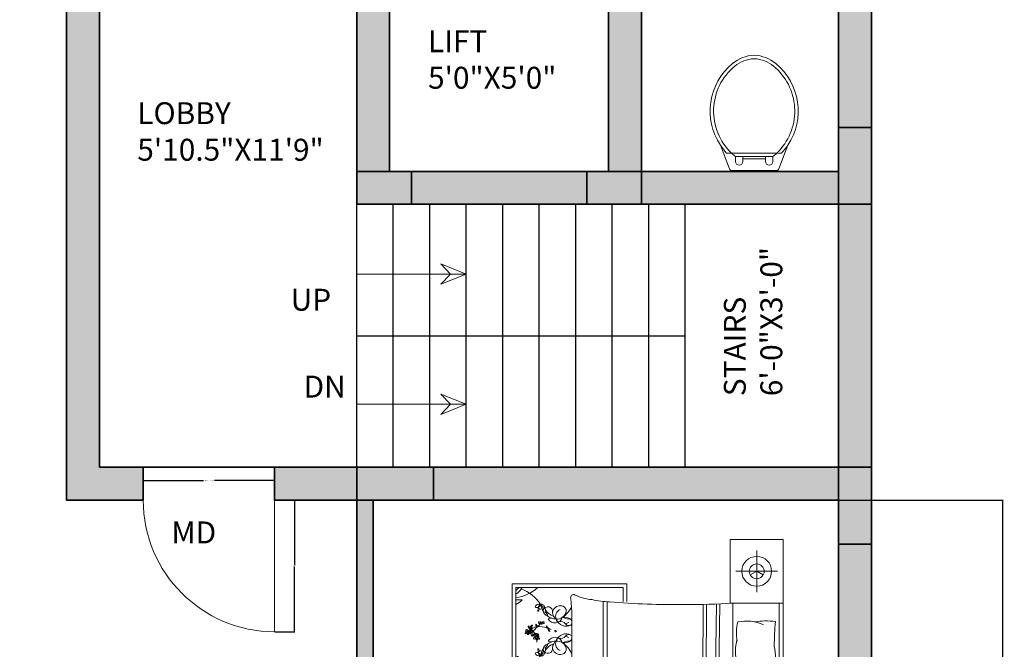
# Model space of a CAD drawing. Units: inches. Extents: x -9 to 505, y -680 to 48.
# Tile 6 of 17: x 235 to 505, y -487 to -314. Entities that reach past the tile are written whole.
import ezdxf

# ---------------------------------------------------------------- set-up
doc = ezdxf.new("R2010")
doc.units = ezdxf.units.IN
doc.header["$MEASUREMENT"] = 0
for name, color, linetype, lineweight in [('A-ANNO-DIMS', 2, 'Continuous', 18), ('A-ANNO-SYMB', 7, 'Continuous', 18), ('A-ANNO-TEXT', 7, 'Continuous', 18), ('A-AREA-IDEN', 7, 'Continuous', 18), ('A-DOOR', 3, 'Continuous', 18), ('A-FLOR-STRS', 7, 'Continuous', 25), ('A-FURN', 8, 'Continuous', 18), ('A-WALL', 7, 'Continuous', 35), ('A-WALL-PATT', 251, 'Continuous', 13), ('S-CONC', 7, 'Continuous', 35), ('S-CONC-PATT', 18, 'Continuous', 13), ('WC-Detail_dwgmodels.com', 251, 'Continuous', 13), ('WC-Outline_dwgmodels.com', 250, 'Continuous', 18)]:
    doc.layers.add(name, color=color, linetype=linetype, lineweight=lineweight)
doc.styles.get("Standard").update_dxf_attribs({"font": 'arial.ttf'})
doc.dimstyles.get("Standard").update_dxf_attribs({"dimtxt": 0.18, "dimasz": 0.18, "dimexe": 0.18, "dimexo": 0.0625, "dimgap": 0.09, "dimtad": 0, "dimtih": 1, "dimtoh": 1, "dimdec": 0, "dimzin": 0, "dimdsep": 46, "dimlunit": 3, "dimtxsty": 'Standard', "dimcen": 0.09, "dimadec": 0, "dimazin": 0, "dimtfac": 1, "dimtdec": 0, "dimtofl": 0, "dimtmove": 0, "dimatfit": 3, "dimfxl": 1, "dimtolj": 1, "dimtzin": 0, "dimarcsym": 0})

# ---------------------------------------------------------------- blocks, each defined once
blk = doc.blocks.new('BED-DOUBLE-WITH-NIGHTSTANDS')
for p, q in [((74.3, 0), (74.3, 87.37)), ((67.02, 72.93), (67.02, 84.34)), ((61.31, 78.63), (72.73, 78.63)), ((0, 75.23), (0, 11.53)), ((31.47, 75.23), (0, 75.23)), ((1.01, 74.22), (30.46, 74.22)), ((1.01, 12.54), (1.01, 74.22)), ((30.46, 74.22), (30.46, 70.37)), ((31.47, 70.38), (31.47, 75.23)), ((24.93, 70.38), (24.93, 16.47)), ((26.02, 70.29), (26.02, 16.47)), ((52.32, 69.59), (52.18, 36.06)), ((53.22, 69.58), (53.09, 36.41)), ((55.97, 69.63), (55.52, 37.9)), ((56.87, 69.66), (56.43, 38.56)), ((60.5, 17.47), (60.5, 69.9)), ((73.18, 69.9), (73.18, 17.47)), ((9.87, 65.61), (10.86, 65.8)), ((9.87, 59.5), (10.86, 59.31)), ((16.35, 61.42), (16.35, 25.95)), ((60.5, 41.48), (53.83, 36.69)), ((57.9, 29.61), (60.5, 39.14)), ((53.83, 36.69), (48.7, 34.74)), ((48.7, 34.74), (46.4, 34.39)), ((46.4, 34.39), (47.11, 31.56)), ((47.11, 31.56), (48.17, 29.26)), ((9.87, 27.26), (10.86, 27.45)), ((48.17, 29.26), (48.7, 25.36)), ((55.6, 23.24), (57.9, 29.61)), ((48.7, 25.36), (49.06, 20.94)), ((53.12, 19.88), (55.6, 23.24)), ((9.87, 21.15), (10.86, 20.96)), ((49.06, 20.94), (48.7, 17.4)), ((49.41, 16.69), (53.12, 19.88)), ((30.46, 16.47), (30.46, 12.54)), ((31.47, 11.53), (31.47, 16.47)), ((48.7, 17.4), (49.41, 16.69)), ((74.3, 17.47), (50.32, 17.47)), ((67.02, 14.45), (67.02, 3.03)), ((0, 11.53), (31.47, 11.53)), ((30.46, 12.54), (1.01, 12.54)), ((61.31, 8.74), (72.73, 8.74))]:
    blk.add_line(p, q)
for points in [[(74.3, 69.9), (59.74, 69.9), (59.74, 87.37), (74.3, 87.37)], [(67.02, 78.63), (65.26, 77.62)], [(67.02, 78.63), (68.79, 77.62)], [(59.74, 17.47), (59.74, 0), (74.3, 0)], [(67.02, 8.74), (65.26, 9.76)], [(67.02, 8.74), (68.79, 9.76)]]:
    blk.add_lwpolyline(points)
for points in [[(26.71, 70.27, -0.056112), (21.91, 70.9, -0.095341), (17.28, 72.13)], [(72.13, 64.88, 0.074897), (66.42, 64.77, -0.472817)], [(66.1, 47.01, 0.14099), (71.92, 46.83, 0.235245)], [(66.1, 43.28, -0.14099), (71.92, 43.45, -0.235245)], [(72.13, 22.49, -0.074897), (66.42, 22.6, 0.472817)], [(41.41, 16.51, -0.001242), (24.83, 16.47, 0.127202), (16.57, 14.72)]]:
    blk.add_lwpolyline(points, format="xyb")
for centre, radius in [((67.02, 78.63), 4.08), ((67.02, 78.63), 2.04), ((4.36, 62.02), 0.223), ((6.7, 60.56), 0.223), ((4.36, 24.75), 0.223), ((6.7, 26.2), 0.223), ((67.02, 8.74), 4.08), ((67.02, 8.74), 2.04)]:
    blk.add_circle(centre, radius)
for centre, radius, start, end in [((-2.05, 76.99), 5.56, 303.4617, 330.1116), ((-3.09, 78.99), 6.93, 306.3036, 316.4814), ((-0.53, 82.71), 11.41, 277.745, 311.8856), ((-1.65, 63.19), 11.41, 34.3865, 68.5908), ((-0.77, 73.87), 4.64, 292.5547, 318.9546), ((1.73, 86.58), 15.79, 267.4081, 273.6519), ((16.83, 71.47), 0.796, 56.1736, 203.4781), ((-68.63, 64.1), 85.02, 358.1965, 4.7598), ((44.11, 274.32), 204.79, 265.1265, 270.8855), ((7.49, 68.4), 1.27, 77.7115, 159.0387), ((6.81, 69.66), 0.953, 238.4633, 358.2869), ((9.93, 67.74), 2.89, 138.8402, 177.9352), ((7.19, 67.84), 0.142, 177.9352, 11.4834), ((7.26, 67.85), 0.0688, 11.4834, 127.9409), ((8.2, 68.81), 0.933, 117.6827, 223.7762), ((7.66, 68.26), 0.0744, 223.7729, 159.7333), ((7.99, 68.72), 0.946, 2.9516, 103.728), ((15.55, 71.37), 7.98, 192.5173, 207.1824), ((6.71, 68.17), 1.8, 345.4653, 54.2343), ((9.43, 70.65), 1.95, 211.3827, 255.2969), ((9.8, 67.61), 1.31, 350.264, 160.8688), ((10.19, 67.92), 1.64, 175.969, 254.3045), ((8.38, 67.88), 0.804, 333.9755, 53.2681), ((8.02, 66.16), 1.74, 6.1662, 51.5825), ((12.69, 70.21), 4.12, 211.2614, 251.7045), ((13.16, 67.13), 2.09, 84.9449, 172.8857), ((13.96, 66.31), 2.03, 111.5819, 201.4221), ((12.28, 68.18), 2.63, 265.2933, 346.921), ((13.37, 67.73), 1.48, 354.4856, 91.0538), ((10.2, 71.58), 6.61, 303.6671, 336.3547), ((49.82, 226.53), 156.99, 269.0718, 273.9), ((7.61, 64.57), 0.367, 127.7621, 169.0403), ((8.1, 64.17), 0.676, 113.4276, 137.6104), ((8.03, 64.87), 0.223, 183.2768, 356.7232), ((8.24, 64.61), 0.213, 1.1081, 91.8675), ((8.37, 64.57), 0.371, 11.5637, 52.6358), ((12.35, 70.24), 4.69, 236.2883, 266.5076), ((11.75, 66.69), 2.17, 209.9085, 343.1337), ((13.63, 67.49), 2.54, 182.3591, 234.0401), ((12.67, 65.32), 0.542, 167.3041, 285.1471), ((14.13, 62.72), 3.37, 122.7011, 126.3445), ((14.77, 66.35), 2.78, 199.2822, 299.1751), ((13.28, 63.06), 1.79, 41.5653, 105.1471), ((15.71, 69.16), 3.62, 238.8218, 280.751), ((14.13, 62.72), 3.37, 55.785, 94.7304), ((15.39, 64.67), 1.05, 17.4186, 52.325), ((73.15, 61.76), 11.71, 165.1039, 191.0369), ((64.13, 53.75), 11.26, 65.1316, 101.7583), ((903.62, 16.72), 832.89, 176.68521, 177.14978), ((3.95, 61.71), 0.367, 61.2196, 169.0403), ((4.19, 62.47), 0.439, 157.4086, 261.4386), ((3.94, 62.48), 0.22, 58.0499, 135.6268), ((4.17, 62.34), 0.147, 172.906, 277.132), ((3.69, 62.07), 0.702, 14.7558, 58.0499), ((4.67, 62.26), 0.303, 36.1046, 181.4281), ((4.68, 63.45), 0.248, 124.3538, 214.3923), ((5.05, 63.41), 0.579, 190.3057, 287.1958), ((4.49, 62.5), 0.306, 270.0645, 331.1507), ((4.75, 62.43), 0.35, 221.8413, 265.7877), ((5.21, 63.62), 0.673, 176.9701, 248.2913), ((10.01, 67.17), 6.5, 212.6784, 216.3746), ((4.75, 62.29), 0.218, 263.7526, 41.7054), ((4.7, 61.71), 0.371, 11.5637, 86.365), ((4.99, 63.46), 0.257, 216.3746, 291.7548), ((7.26, 59.85), 3.63, 124.0033, 132.4917), ((3.53, 59.39), 3.88, 63.7819, 68.2913), ((5.6, 62.38), 0.616, 128.3208, 208.8162), ((5.6, 63.28), 0.579, 122.8155, 187.3992), ((5.71, 62.42), 0.737, 207.7043, 254.3516), ((5.16, 63.04), 0.194, 289.3605, 111.7548), ((5.3, 63.04), 0.194, 221.8703, 44.2646), ((6.18, 62.48), 1.01, 157.2305, 229.0635), ((5.86, 63.21), 0.673, 109.4799, 177.6828), ((5.84, 62.81), 0.597, 174.4544, 220.6188), ((2.45, 59.48), 4.35, 30.544, 49.818), ((5.5, 63.63), 0.248, 56.8636, 146.9021), ((5.62, 63.36), 0.257, 148.8844, 224.2646), ((4.84, 61.96), 0.717, 340.0041, 40.6188), ((10.97, 60.13), 6.5, 145.1882, 148.8844), ((7.26, 59.85), 3.63, 94.756, 119.2041), ((14.99, 54.63), 11.94, 132.2412, 142.1744), ((8.96, 64.13), 2.46, 178.3264, 187.1302), ((6.3, 63.79), 0.459, 11.3256, 64.4621), ((7.86, 64.45), 1.38, 190.2588, 210.656), ((6.93, 63.89), 0.419, 188.3432, 274.2869), ((7.3, 64.12), 0.732, 210.656, 242.6341), ((7.85, 64.75), 1.4, 218.2101, 226.3071), ((6.82, 63.57), 0.178, 325.7657, 67.4417), ((1.29, 69.52), 8.3, 313.1541, 322.0459), ((7.45, 56.25), 7.24, 73.5842, 93.8277), ((7.39, 64.54), 0.171, 142.4737, 265.053), ((7.42, 64.88), 0.517, 265.053, 338.3618), ((8.19, 64.47), 0.364, 139.7889, 227.6792), ((8.07, 64.34), 0.192, 227.6792, 350.3487), ((7.33, 64.48), 0.728, 353.0852, 15.7171), ((7.81, 64.39), 0.46, 350.3487, 43.6538), ((8.66, 64.86), 0.535, 198.7263, 262.5032), ((8.64, 64.5), 0.172, 255.2356, 54.9248), ((11.9, 63.61), 2.46, 178.3264, 187.1302), ((9.24, 63.27), 0.459, 11.3256, 64.4621), ((10.8, 63.93), 1.38, 190.2588, 210.656), ((9.87, 63.37), 0.419, 188.3432, 274.2869), ((10.24, 63.6), 0.732, 210.656, 242.6341), ((10.79, 64.23), 1.4, 218.2101, 226.3071), ((9.76, 63.05), 0.178, 325.7657, 67.4417), ((10.26, 62.72), 0.419, 147.5332, 233.4768), ((10.63, 62.94), 0.732, 179.1859, 211.164), ((9.92, 62.77), 0.178, 354.3784, 96.0543), ((7.45, 56.25), 7.24, 63.0032, 69.8941), ((11.19, 63.27), 1.38, 211.164, 231.5612), ((11.43, 64.4), 2.46, 234.6898, 243.4936), ((11.45, 63.13), 1.4, 195.5129, 203.6099), ((9.87, 62.21), 0.459, 357.3579, 50.4944), ((11.84, 62.3), 0.168, 12.7051, 190.4384), ((11.95, 62.32), 0.274, 190.4384, 10.4136), ((14.26, 66.77), 2.51, 277.436, 299.9149), ((15.59, 65.12), 1.31, 221.5653, 293.8354), ((15.39, 64.67), 1.05, 314.4517, 343.3657), ((3.72, 61.68), 0.171, 142.4737, 265.053), ((3.75, 62.02), 0.517, 265.053, 338.3618), ((4.44, 61.32), 0.676, 113.4276, 137.6104), ((4.52, 61.61), 0.364, 139.7889, 227.6792), ((4.41, 61.49), 0.192, 227.6792, 350.3487), ((3.66, 61.62), 0.728, 353.0852, 15.7171), ((4.14, 61.53), 0.46, 350.3487, 43.6538), ((4.99, 62.01), 0.535, 198.7263, 262.5032), ((4.57, 61.76), 0.213, 1.1081, 91.8675), ((4.97, 61.64), 0.172, 255.2356, 54.9248), ((5.23, 62), 1.01, 270.278, 342.111), ((5.91, 60.73), 0.717, 98.7227, 159.3375), ((5.55, 61.65), 0.737, 244.9899, 291.6373), ((5.71, 62.03), 0.597, 278.7227, 324.8872), ((5.61, 61.55), 0.616, 290.5253, 358.5375), ((6.07, 60.22), 0.171, 142.4737, 265.053), ((6.29, 60.26), 0.367, 61.2196, 169.0403), ((6.1, 60.57), 0.517, 265.053, 338.3618), ((6.53, 61.01), 0.439, 157.4086, 261.4386), ((6.29, 61.03), 0.22, 58.0499, 135.6268), ((6.81, 61.72), 0.616, 182.8499, 266.1226), ((6.57, 62.16), 0.597, 231.7607, 277.9252), ((7.04, 62.26), 1.01, 214.5369, 286.3699), ((6.78, 59.86), 0.676, 113.4276, 137.6104), ((6.52, 60.89), 0.147, 172.906, 277.132), ((6.03, 60.62), 0.702, 14.7558, 58.0499), ((2.45, 59.48), 4.35, 23.0501, 23.8477), ((6.87, 60.16), 0.364, 139.7889, 227.6792), ((6.75, 60.03), 0.192, 227.6792, 350.3487), ((6.75, 60.86), 0.717, 37.3105, 97.9252), ((7.01, 60.81), 0.303, 36.1046, 181.4281), ((6.01, 60.16), 0.728, 353.0852, 15.7171), ((6.83, 61.84), 0.737, 265.0106, 311.658), ((2.45, 59.48), 4.35, 357.1071, 4.7585), ((6.49, 60.07), 0.46, 350.3487, 43.6538), ((7.34, 60.55), 0.535, 198.7263, 262.5032), ((6.84, 61.04), 0.306, 270.0645, 331.1507), ((7.1, 60.97), 0.35, 221.8413, 265.7877), ((6.91, 60.3), 0.213, 1.1081, 91.8675), ((7.1, 60.84), 0.218, 263.7526, 41.7054), ((7.05, 60.25), 0.371, 11.5637, 86.365), ((7.31, 60.19), 0.172, 255.2356, 54.9248), ((12.35, 54.86), 4.69, 93.4924, 123.7117), ((11.75, 58.42), 2.17, 16.8663, 150.0915), ((13.63, 57.62), 2.54, 125.9599, 177.6409), ((13.96, 58.8), 2.03, 158.5779, 248.4181), ((12.28, 56.93), 2.63, 13.079, 94.7067), ((12.67, 59.79), 0.542, 74.8529, 192.6959), ((14.77, 58.76), 2.78, 60.8249, 160.7178), ((14.13, 62.39), 3.37, 233.6555, 237.2989), ((13.28, 62.05), 1.79, 254.8529, 318.4347), ((15.71, 55.95), 3.62, 79.7133, 121.1782), ((14.13, 62.39), 3.37, 265.2696, 304.215), ((14.26, 58.33), 2.51, 60.0851, 82.564), ((15.59, 59.99), 1.31, 66.1646, 138.4347), ((15.39, 60.44), 1.05, 307.675, 336.7144), ((15.39, 60.44), 1.05, 23.2856, 45.5483), ((72.29, 56.71), 11.12, 163.8254, 206.1239), ((7.19, 57.27), 0.142, 348.5166, 182.0648), ((9.93, 57.37), 2.89, 182.0648, 221.1598), ((7.26, 57.26), 0.0688, 232.0591, 348.5166), ((8.2, 56.3), 0.933, 136.2238, 242.3173), ((7.61, 56.86), 0.123, 200.2817, 136.2238), ((6.71, 56.94), 1.8, 305.7657, 14.5347), ((15.55, 53.74), 7.98, 152.8176, 167.4827), ((10.19, 57.19), 1.64, 105.6955, 184.031), ((9.8, 57.5), 1.31, 199.1312, 9.736), ((8.38, 57.23), 0.804, 306.7319, 26.0245), ((8.02, 58.95), 1.74, 308.4175, 353.8338), ((12.69, 54.9), 4.12, 108.2955, 148.7386), ((13.16, 57.98), 2.09, 187.1143, 275.0551), ((13.37, 57.38), 1.48, 268.9462, 5.5144), ((10.2, 53.53), 6.61, 21.4941, 56.3329), ((56.84, 54.51), 15.36, 348.8159, 13.6573), ((-0.77, 51.23), 4.64, 41.0454, 67.4453), ((1.73, 38.53), 15.79, 86.3481, 92.5919), ((-1.65, 61.92), 11.41, 291.4092, 325.6135), ((6.81, 55.44), 0.953, 1.7131, 121.5367), ((7.49, 56.71), 1.27, 200.9613, 282.2885), ((7.99, 56.39), 0.946, 256.272, 357.0484), ((9.43, 54.46), 1.95, 104.7031, 148.6173), ((2.11, 44.94), 8.83, 8.1803, 97.1364), ((1.49, 50.77), 2.05, 10.9261, 103.6102), ((1.78, 49.23), 2.59, 48.0951, 107.1391), ((-6.64, 46.18), 11.41, 4.4623, 27.4146), ((-4.99, 49.37), 6.27, 343.5431, 17.0202), ((2.92, 46.08), 5.11, 83.3805, 111.883), ((66.26, 48.62), 4.63, 161.4593, 204.9817), ((67.77, 48.03), 4.32, 343.8974, 26.6563), ((-8.22, 46.89), 9.28, 4.3787, 5.6357), ((-14.58, 42), 16.58, 19.7217, 19.9028), ((3.89, 46.13), 1.27, 47.7873, 129.1145), ((3.93, 47.57), 0.953, 208.5391, 328.3627), ((3.35, 45.79), 0.142, 148.011, 341.5592), ((5.67, 44.34), 2.89, 108.9159, 148.011), ((4.7, 46.14), 0.933, 87.7585, 193.852), ((3.96, 45.93), 0.0744, 193.9791, 129.8091), ((12.35, 44.68), 7.98, 162.593, 177.2582), ((3.09, 46.33), 1.8, 315.5411, 24.3101), ((6.69, 47.12), 1.95, 181.4585, 225.3727), ((4.47, 46.16), 0.946, 333.0274, 73.8037), ((10, 45.26), 1.27, 47.7873, 129.1145), ((10.04, 46.7), 0.953, 208.5391, 328.3627), ((11.79, 43.47), 2.89, 108.9159, 148.011), ((10.81, 45.26), 0.933, 87.7585, 193.852), ((9.21, 45.45), 1.8, 315.5411, 24.3101), ((18.47, 43.81), 7.98, 162.593, 177.2582), ((10.59, 45.29), 0.946, 333.0274, 73.8037), ((12.8, 46.25), 1.95, 181.4585, 225.3727), ((63.18, 57.31), 10.71, 264.0129, 285.8293), ((-0.53, 44.37), 11.41, 277.745, 355.5377), ((3.35, 43.88), 0.142, 18.4408, 211.989), ((5.67, 45.33), 2.89, 211.989, 251.0841), ((3.42, 45.77), 0.0688, 341.5592, 98.0167), ((3.42, 43.9), 0.0688, 261.9833, 18.4408), ((4.7, 43.54), 0.933, 166.148, 272.2415), ((3.92, 43.73), 0.123, 230.0755, 166.148), ((12.35, 44.99), 7.98, 182.7418, 197.407), ((3.09, 43.35), 1.8, 335.6899, 44.4589), ((6.69, 42.55), 1.95, 134.6273, 178.5415), ((4.47, 43.51), 0.946, 286.1963, 26.9726), ((10.04, 42.98), 0.953, 31.6373, 151.4609), ((10, 44.41), 1.27, 230.8855, 312.2127), ((9.46, 44.92), 0.142, 148.011, 341.5592), ((9.46, 44.75), 0.142, 18.4408, 211.989), ((11.79, 46.21), 2.89, 211.989, 251.0841), ((9.53, 44.9), 0.0688, 341.5592, 98.0167), ((9.53, 44.78), 0.0688, 261.9833, 18.4408), ((10.81, 44.41), 0.933, 166.148, 272.2415), ((10.03, 44.6), 0.123, 230.0755, 166.148), ((10.07, 45.06), 0.0744, 193.9791, 129.8091), ((9.21, 44.22), 1.8, 335.6899, 44.4589), ((18.47, 45.87), 7.98, 182.7418, 197.407), ((10.59, 44.39), 0.946, 286.1963, 26.9726), ((12.8, 43.43), 1.95, 134.6273, 178.5415), ((77.04, 40), 15.41, 166.3762, 190.1383), ((63.18, 32.98), 10.71, 74.1707, 95.9871), ((56.52, 41.16), 15.57, 346.04, 8.4751), ((-4.99, 40.3), 6.27, 342.9798, 16.4569), ((-8.22, 42.79), 9.28, 354.3643, 355.6213), ((-14.58, 47.67), 16.58, 340.0972, 340.2783), ((3.93, 42.1), 0.953, 31.6373, 151.4609), ((3.89, 43.54), 1.27, 230.8855, 312.2127), ((-6.64, 43.49), 11.41, 332.5854, 355.5377), ((-2.05, 38.64), 5.56, 303.4617, 358.728), ((-5.04, 44.28), 10.31, 305.947, 325.9877), ((-3.09, 40.64), 6.93, 306.3036, 342.1496), ((81.47, 31.77), 20.31, 160.7385, 191.9603), ((40.51, 34.46), 31.69, 350.503, 7.7804), ((-1.65, 24.85), 11.41, 34.3865, 68.5908), ((1.73, 48.24), 15.79, 267.4081, 273.6519), ((-0.77, 35.53), 4.64, 292.5547, 318.9546), ((46.33, 34.19), 0.211, 70.2464, 181.1377), ((79.42, 40.46), 33.88, 190.6617, 199.8806), ((7.49, 30.05), 1.27, 77.7115, 159.0387), ((6.81, 31.32), 0.953, 238.4633, 358.2869), ((9.93, 29.39), 2.89, 138.8402, 177.9352), ((8.2, 30.46), 0.933, 117.6827, 223.7762), ((7.66, 29.92), 0.0744, 223.7729, 159.7333), ((7.99, 30.37), 0.946, 2.9516, 103.728), ((9.43, 32.3), 1.95, 211.3827, 255.2969), ((6.71, 29.83), 1.8, 345.4653, 54.2343), ((15.55, 33.02), 7.98, 192.5173, 207.1824), ((9.8, 29.26), 1.31, 350.264, 160.8688), ((10.19, 29.57), 1.64, 175.969, 254.3045), ((8.38, 29.53), 0.804, 333.9755, 53.2681), ((12.69, 31.86), 4.12, 211.2614, 251.7045), ((13.16, 28.78), 2.09, 84.9449, 172.8857), ((13.96, 27.96), 2.03, 111.5819, 201.4221), ((13.37, 29.38), 1.48, 354.4856, 91.0538), ((10.2, 33.24), 6.61, 303.6671, 338.5059), ((2.45, 27.28), 4.35, 355.2415, 2.8929), ((7.19, 29.49), 0.142, 177.9352, 11.4834), ((7.26, 29.5), 0.0688, 11.4834, 127.9409), ((8.02, 27.81), 1.74, 6.1662, 51.5825), ((12.35, 31.9), 4.69, 236.2883, 266.5076), ((11.75, 28.34), 2.17, 209.9085, 343.1337), ((13.63, 29.14), 2.54, 182.3591, 234.0401), ((12.28, 29.84), 2.63, 265.2933, 346.921), ((12.67, 26.97), 0.542, 167.3041, 285.1471), ((14.13, 24.37), 3.37, 122.7011, 126.3445), ((14.77, 28.01), 2.78, 199.2822, 299.1751), ((15.71, 30.81), 3.62, 238.8218, 280.2867), ((14.13, 24.37), 3.37, 55.785, 94.7304), ((15.39, 26.33), 1.05, 23.2856, 52.325), ((41.05, 26.07), 7.11, 348.6608, 23.7384), ((73.15, 25.61), 11.71, 168.9631, 194.8961), ((903.62, 70.65), 832.89, 182.85022, 183.31479), ((3.72, 25.08), 0.171, 94.947, 217.5263), ((3.95, 25.05), 0.367, 190.9597, 298.7804), ((3.75, 24.74), 0.517, 21.6382, 94.947), ((4.19, 24.29), 0.439, 98.5614, 202.5914), ((4.44, 25.45), 0.676, 222.3896, 246.5724), ((4.17, 24.42), 0.147, 82.868, 187.094), ((3.69, 24.69), 0.702, 301.9501, 345.2442), ((4.52, 25.15), 0.364, 132.3208, 220.2111), ((4.41, 25.28), 0.192, 9.6513, 132.3208), ((3.66, 25.14), 0.728, 344.2829, 6.9148), ((4.67, 24.5), 0.303, 178.5719, 323.8954), ((4.14, 25.23), 0.46, 316.3462, 9.6513), ((4.99, 24.76), 0.535, 97.4968, 161.2737), ((4.75, 24.34), 0.35, 94.2123, 138.1587), ((4.49, 24.26), 0.306, 28.8493, 89.9355), ((4.57, 25.01), 0.213, 268.1325, 358.8919), ((4.7, 25.05), 0.371, 273.635, 348.4363), ((4.75, 24.47), 0.218, 318.2946, 96.2474), ((4.97, 25.12), 0.172, 305.0752, 104.7644), ((5.6, 24.39), 0.616, 151.1838, 231.6792), ((5.71, 24.34), 0.737, 105.6484, 152.2957), ((6.18, 24.28), 1.01, 130.9365, 202.7695), ((5.55, 25.11), 0.737, 68.3627, 115.0101), ((5.23, 24.76), 1.01, 17.889, 89.722), ((5.91, 26.03), 0.717, 200.6625, 261.2773), ((5.84, 23.95), 0.597, 139.3812, 185.5456), ((2.45, 27.28), 4.35, 310.182, 329.456), ((4.84, 24.8), 0.717, 319.3812, 19.9959), ((14.99, 32.13), 11.94, 217.8256, 227.7588), ((5.71, 24.73), 0.597, 35.1128, 81.2773), ((5.61, 25.22), 0.616, 1.4625, 69.4747), ((6.07, 26.54), 0.171, 94.947, 217.5263), ((6.29, 26.51), 0.367, 190.9597, 298.7804), ((6.1, 26.19), 0.517, 21.6382, 94.947), ((6.53, 25.75), 0.439, 98.5614, 202.5914), ((6.29, 25.74), 0.22, 224.3732, 301.9501), ((6.81, 25.04), 0.616, 93.8774, 177.1501), ((7.04, 24.5), 1.01, 73.6301, 145.4631), ((6.57, 24.61), 0.597, 82.0748, 128.2393), ((6.78, 26.9), 0.676, 222.3896, 246.5724), ((6.52, 25.87), 0.147, 82.868, 187.094), ((6.03, 26.14), 0.702, 301.9501, 345.2442), ((2.45, 27.28), 4.35, 336.1523, 336.9499), ((6.87, 26.61), 0.364, 132.3208, 220.2111), ((6.75, 26.73), 0.192, 9.6513, 132.3208), ((6.75, 25.91), 0.717, 262.0748, 322.6895), ((6.01, 26.6), 0.728, 344.2829, 6.9148), ((7.01, 25.96), 0.303, 178.5719, 323.8954), ((6.83, 24.92), 0.737, 48.342, 94.9894), ((6.49, 26.69), 0.46, 316.3462, 9.6513), ((7.34, 26.21), 0.535, 97.4968, 161.2737), ((7.1, 25.79), 0.35, 94.2123, 138.1587), ((6.84, 25.72), 0.306, 28.8493, 89.9355), ((6.91, 26.46), 0.213, 268.1325, 358.8919), ((7.05, 26.51), 0.371, 273.635, 348.4363), ((7.1, 25.92), 0.218, 318.2946, 96.2474), ((7.31, 26.58), 0.172, 305.0752, 104.7644), ((10.26, 24.04), 0.419, 126.5232, 212.4668), ((11.19, 23.49), 1.38, 128.4388, 148.836), ((11.43, 22.37), 2.46, 116.5064, 125.3102), ((9.87, 24.55), 0.459, 309.5056, 2.6421), ((11.95, 24.44), 0.274, 349.5864, 169.5616), ((11.84, 24.46), 0.168, 169.5616, 347.2949), ((13.28, 24.72), 1.79, 41.5653, 105.1471), ((14.26, 28.43), 2.51, 277.436, 299.9149), ((15.59, 26.77), 1.31, 221.5653, 293.8354), ((-74.6, 24.91), 90.96, 354.3113, 0.6567), ((15.39, 26.33), 1.05, 314.4517, 336.771), ((80.35, 18.19), 32.98, 168.6608, 182.5481), ((3.94, 24.28), 0.22, 224.3732, 301.9501), ((4.68, 23.31), 0.248, 145.6077, 235.6462), ((5.05, 23.35), 0.579, 72.8042, 169.6943), ((5.21, 23.14), 0.673, 111.7087, 183.0299), ((10.01, 19.6), 6.5, 143.6254, 147.3216), ((4.99, 23.3), 0.257, 68.2452, 143.6254), ((7.26, 26.91), 3.63, 227.5083, 235.9967), ((3.53, 27.37), 3.88, 291.7087, 296.2181), ((5.6, 23.48), 0.579, 172.6008, 237.1845), ((5.16, 23.72), 0.194, 248.2452, 70.6395), ((5.3, 23.72), 0.194, 315.7354, 138.1297), ((5.86, 23.55), 0.673, 182.3172, 250.5201), ((5.5, 23.13), 0.248, 213.0979, 303.1364), ((5.62, 23.4), 0.257, 135.7354, 211.1156), ((10.97, 26.63), 6.5, 211.1156, 214.8118), ((7.26, 26.91), 3.63, 240.7959, 265.244), ((7.86, 22.31), 1.38, 149.344, 169.7412), ((8.96, 22.63), 2.46, 172.8698, 181.6736), ((6.3, 22.97), 0.459, 295.5379, 348.6744), ((6.93, 22.88), 0.419, 85.7131, 171.6568), ((7.3, 22.64), 0.732, 117.3659, 149.344), ((7.85, 22.01), 1.4, 133.6929, 141.7899), ((6.82, 23.19), 0.178, 292.5583, 34.2343), ((7.45, 30.51), 7.24, 266.1723, 286.4158), ((1.29, 17.24), 8.3, 37.9541, 46.8459), ((7.39, 22.23), 0.171, 94.947, 217.5263), ((7.61, 22.19), 0.367, 190.9597, 232.2379), ((7.42, 21.88), 0.517, 21.6382, 94.947), ((8.1, 22.59), 0.676, 222.3896, 246.5724), ((8.03, 21.89), 0.223, 3.2768, 176.7232), ((8.19, 22.29), 0.364, 132.3208, 220.2111), ((8.07, 22.42), 0.192, 9.6513, 132.3208), ((7.33, 22.29), 0.728, 344.2829, 6.9148), ((7.81, 22.37), 0.46, 316.3462, 9.6513), ((8.66, 21.9), 0.535, 97.4968, 161.2737), ((8.24, 22.15), 0.213, 268.1325, 358.8919), ((8.64, 22.26), 0.172, 305.0752, 104.7644), ((8.37, 22.2), 0.371, 307.3642, 348.4363), ((10.8, 22.83), 1.38, 149.344, 169.7412), ((11.9, 23.15), 2.46, 172.8698, 181.6736), ((9.24, 23.49), 0.459, 295.5379, 348.6744), ((9.87, 23.4), 0.419, 85.7131, 171.6568), ((10.24, 23.16), 0.732, 117.3659, 149.344), ((10.79, 22.54), 1.4, 133.6929, 141.7899), ((9.76, 23.71), 0.178, 292.5583, 34.2343), ((11.75, 20.07), 2.17, 16.8663, 150.0915), ((10.63, 23.83), 0.732, 148.836, 180.8141), ((9.92, 23.99), 0.178, 263.9457, 5.6216), ((7.45, 30.51), 7.24, 290.1059, 296.9968), ((11.45, 23.63), 1.4, 156.3901, 164.4871), ((12.67, 21.45), 0.542, 74.8529, 192.6959), ((14.77, 20.41), 2.78, 60.8249, 160.7178), ((13.28, 23.7), 1.79, 254.8529, 318.4347), ((14.26, 19.99), 2.51, 60.0851, 82.564), ((15.59, 21.64), 1.31, 66.1646, 138.4347), ((15.39, 22.09), 1.05, 26.442, 45.5483), ((64.13, 33.62), 11.26, 258.2417, 294.8684), ((7.19, 18.93), 0.142, 348.5166, 182.0648), ((9.93, 19.03), 2.89, 182.0648, 221.1598), ((7.26, 18.91), 0.0688, 232.0591, 348.5166), ((15.55, 15.4), 7.98, 152.8176, 167.4827), ((6.71, 18.59), 1.8, 305.7657, 14.5347), ((10.19, 18.84), 1.64, 105.6955, 184.031), ((9.8, 19.16), 1.31, 199.1312, 9.736), ((8.38, 18.89), 0.804, 306.7319, 26.0245), ((8.02, 20.61), 1.74, 308.4175, 353.8338), ((12.69, 16.56), 4.12, 108.2955, 148.7386), ((12.35, 16.52), 4.69, 93.4924, 123.7117), ((13.63, 19.27), 2.54, 125.9599, 177.6409), ((13.16, 19.64), 2.09, 187.1143, 275.0551), ((13.96, 20.46), 2.03, 158.5779, 248.4181), ((12.28, 18.58), 2.63, 13.079, 94.7067), ((14.13, 24.04), 3.37, 233.6555, 237.2989), ((13.37, 19.03), 1.48, 268.9462, 5.5144), ((15.71, 17.61), 3.62, 80.8446, 121.1782), ((14.13, 24.04), 3.37, 265.2696, 304.215), ((10.2, 15.18), 6.61, 26.7003, 56.3329), ((15.39, 22.09), 1.05, 307.675, 329.9707), ((-0.77, 12.89), 4.64, 41.0454, 67.4453), ((-1.65, 23.57), 11.41, 291.4092, 325.6135), ((6.81, 17.1), 0.953, 1.7131, 121.5367), ((7.49, 18.36), 1.27, 200.9613, 282.2885), ((8.2, 17.95), 0.933, 136.2238, 242.3173), ((7.61, 18.51), 0.123, 200.2817, 136.2238), ((9.43, 16.11), 1.95, 104.7031, 148.6173), ((7.99, 18.05), 0.946, 256.272, 357.0484), ((47.24, -63.42), 80.14, 88.447, 94.1706), ((1.73, 0.18), 15.79, 86.3481, 92.5919), ((-0.53, 4.05), 11.41, 48.1144, 82.255), ((-2.05, 9.77), 5.56, 29.8884, 56.5383), ((16.63, 15.52), 0.806, 152.6588, 266.02), ((-3.09, 7.77), 6.93, 43.5186, 53.6964)]:
    blk.add_arc(centre, radius, start, end)
blk = doc.blocks.new('STAIR-DIRECTION-ARROW')
for p, q in [((30, 2.8), (23.01, 5.59)), ((23.01, 5.59), (25.65, 2.8)), ((0, 2.8), (30, 2.8)), ((30, 2.8), (23.01, 0)), ((23.01, 0), (25.65, 2.8))]:
    blk.add_line(p, q)
blk = doc.blocks.new('DOOR-ENTRY-36')
blk.add_line((36, 0), (36, 36))
blk.add_arc((36, 0), 36, 90, 180)
blk = doc.blocks.new('*D26')
at = {"layer": 'A-ANNO-DIMS', "color": 0, "lineweight": -2, "transparency": 16777216}
for p, q in [((269.26, -445.94), (269.26, -440.42)), ((269.44, -440.6), (285.76, -440.6)), ((305.08, -440.6), (288.77, -440.6)), ((305.26, -445.94), (305.26, -440.42))]:
    blk.add_line(p, q, dxfattribs=at)
at = {"layer": 'A-ANNO-DIMS', "color": 0, "transparency": 16777216}
for points in [[(269.44, -440.57), (269.44, -440.63), (269.26, -440.6)], [(305.08, -440.57), (305.08, -440.63), (305.26, -440.6)]]:
    blk.add_solid(points, dxfattribs=at)
at = {"layer": 'Defpoints', "color": 0, "transparency": 16777216}
for p in [(305.26, -440.6), (269.26, -446), (305.26, -446)]:
    blk.add_point(p, dxfattribs=at)
at = {"layer": 'A-ANNO-DIMS', "color": 0, "transparency": 16777216, "insert": (287.26, -440.6), "char_height": 0.18, "attachment_point": 5}
blk.add_mtext('\\A1;ENTRY DOOR 3\'-0" TYP.', dxfattribs=at)
blk = doc.blocks.new('*D27')
at = {"layer": 'A-ANNO-DIMS', "color": 0, "lineweight": -2, "transparency": 16777216}
for p, q in [((305.33, -446), (310.84, -446)), ((310.66, -446.18), (310.66, -463.82)), ((310.66, -481.82), (310.66, -464.18)), ((305.33, -482), (310.84, -482))]:
    blk.add_line(p, q, dxfattribs=at)
at = {"layer": 'A-ANNO-DIMS', "color": 0, "transparency": 16777216}
for points in [[(310.63, -446.18), (310.69, -446.18), (310.66, -446)], [(310.63, -481.82), (310.69, -481.82), (310.66, -482)]]:
    blk.add_solid(points, dxfattribs=at)
at = {"layer": 'Defpoints', "color": 0, "transparency": 16777216}
for p in [(305.26, -446), (305.26, -482), (310.66, -482)]:
    blk.add_point(p, dxfattribs=at)
at = {"layer": 'A-ANNO-DIMS', "color": 0, "transparency": 16777216, "insert": (310.66, -464), "char_height": 0.18, "attachment_point": 5}
blk.add_mtext('\\A1;3\'-0" TYP.', dxfattribs=at)
blk = doc.blocks.new('*D48')
at = {"layer": 'A-ANNO-DIMS', "color": 0, "lineweight": -2, "transparency": 16777216}
for p, q in [((459.83, -446), (504.82, -446)), ((504.64, -446.18), (504.64, -562.57)), ((504.64, -679.32), (504.64, -562.93)), ((468.83, -679.5), (504.82, -679.5))]:
    blk.add_line(p, q, dxfattribs=at)
at = {"layer": 'A-ANNO-DIMS', "color": 0, "transparency": 16777216}
for points in [[(504.61, -446.18), (504.67, -446.18), (504.64, -446)], [(504.61, -679.32), (504.67, -679.32), (504.64, -679.5)]]:
    blk.add_solid(points, dxfattribs=at)
at = {"layer": 'Defpoints', "color": 0, "transparency": 16777216}
for p in [(459.76, -446), (468.76, -679.5), (504.64, -679.5)]:
    blk.add_point(p, dxfattribs=at)
at = {"layer": 'A-ANNO-DIMS', "color": 0, "transparency": 16777216, "insert": (504.64, -562.75), "char_height": 0.18, "attachment_point": 5}
blk.add_mtext('\\A1;19\'-5 1/2"', dxfattribs=at)

msp = doc.modelspace()

# ---------------------------------------------------------------- hatches: boundary and pattern name
at = {"layer": 'A-WALL-PATT'}
h = msp.add_hatch(color=256, dxfattribs=at)
h.dxf.hatch_style = 1
h.paths.add_polyline_path([(101.64, 11.5), (48.26, 11.5), (48.26, 2.5), (72.26, 2.5), (72.26, -21.25), (81.26, -21.25), (81.26, 2.5), (101.64, 2.5)])
h.paths.add_polyline_path([(36.26, 2.5), (27.26, 2.5), (27.26, -6.92), (36.26, -6.92)])
h.paths.add_polyline_path([(81.26, -57.25), (72.26, -57.25), (72.26, -75.5), (81.26, -75.5)])
h.paths.add_polyline_path([(162.76, 11.5), (137.64, 11.5), (137.64, 2.5), (162.76, 2.5)])
h.paths.add_polyline_path([(179.26, 2.5), (174.76, 2.5), (174.76, -75.5), (179.26, -75.5), (179.26, -54.5), (229.51, -54.5), (229.51, -45.5), (179.26, -45.5)])
h.paths.add_polyline_path([(382.26, -45.5), (332.26, -45.5), (332.26, 2.5), (327.76, 2.5), (327.76, -45.5), (277.51, -45.5), (277.51, -54.5), (327.76, -54.5), (327.76, -111.5), (332.26, -111.5), (332.26, -54.5), (382.26, -54.5)])
h.paths.add_polyline_path([(332.26, -128), (327.76, -128), (327.76, -207), (332.26, -207)])
h.paths.add_polyline_path([(124.76, -111.5), (36.26, -111.5), (36.26, -116), (120.26, -116), (120.26, -168.5), (179.26, -168.5), (179.26, -164), (124.76, -164)])
h.paths.add_polyline_path([(96.26, -164), (36.26, -164), (36.26, -152), (27.26, -152), (27.26, -208.88), (36.26, -208.88), (36.26, -168.5), (96.26, -168.5)])
h.paths.add_polyline_path([(36.26, -244.88), (27.26, -244.88), (27.26, -287), (36.26, -287)])
h.paths.add_polyline_path([(179.26, -204.5), (174.76, -204.5), (174.76, -287), (179.26, -287)])
h.paths.add_polyline_path([(257.26, -296), (248.26, -296), (248.26, -446), (269.26, -446), (269.26, -437), (257.26, -437)])
h.paths.add_polyline_path([(90.26, -296), (81.26, -296), (81.26, -348.67), (90.26, -348.67)])
h.paths.add_polyline_path([(90.26, -384.67), (81.26, -384.67), (81.26, -416), (90.26, -416)])
h.paths.add_polyline_path([(170.26, -452), (36.26, -452), (36.26, -456.5), (165.76, -456.5), (165.76, -504.5), (165.13, -504.5), (165.13, -509), (170.26, -509)])
h.paths.add_polyline_path([(141.76, -504.5), (36.26, -504.5), (36.26, -492.5), (27.26, -492.5), (27.26, -565.96), (36.26, -565.96), (36.26, -509), (141.76, -509)])
h.paths.add_polyline_path([(36.26, -601.96), (27.26, -601.96), (27.26, -658.5), (36.26, -658.5)])
h.paths.add_polyline_path([(170.26, -670.5), (170.26, -634.5), (222.76, -634.5), (222.76, -625.5), (165.76, -625.5), (165.76, -670.5), (36.26, -670.5), (36.26, -679.5), (170.26, -679.5)])
h.paths.add_polyline_path([(332.26, -616.5), (433.89, -616.5), (433.89, -612), (332.26, -612), (332.26, -610.56), (327.76, -610.56), (327.76, -625.5), (270.76, -625.5), (270.76, -634.5), (327.76, -634.5), (327.76, -658.5), (332.26, -658.5)])
h.paths.add_polyline_path([(459.76, -670.5), (336.76, -670.5), (336.76, -679.5), (459.76, -679.5)])
h.paths.add_polyline_path([(468.76, -545.74), (459.76, -545.74), (459.76, -612), (457.89, -612), (457.89, -616.5), (459.76, -616.5), (459.76, -658.5), (468.76, -658.5)])
h.paths.add_polyline_path([(332.26, -446), (327.76, -446), (327.76, -574.56), (332.26, -574.56)])
h.paths.add_polyline_path([(327.76, -437), (305.26, -437), (305.26, -446), (327.76, -446)])
h.paths.add_polyline_path([(459.76, -437), (348.76, -437), (348.76, -446), (459.76, -446)])
h.paths.add_polyline_path([(468.76, -458), (459.76, -458), (459.76, -509.74), (468.76, -509.74)])
h.paths.add_polyline_path([(468.76, -365), (459.76, -365), (459.76, -437), (468.76, -437)])
h.paths.add_polyline_path([(468.76, -299.6), (459.76, -299.6), (459.76, -344), (468.76, -344)])
h.paths.add_polyline_path([(468.76, -184.74), (459.76, -184.74), (459.76, -231), (401.26, -231), (401.26, -235.5), (459.76, -235.5), (459.76, -275.6), (468.76, -275.6)])
h.paths.add_polyline_path([(390.76, -356), (342.76, -356), (342.76, -365), (390.76, -365)])
h.paths.add_polyline_path([(459.76, -356), (405.76, -356), (405.76, -365), (459.76, -365)])
h.paths.add_polyline_path([(405.76, -296), (396.76, -296), (396.76, -356), (405.76, -356)])
h.paths.add_polyline_path([(336.76, -296), (327.76, -296), (327.76, -356), (336.76, -356)])
h.paths.add_polyline_path([(468.76, -9.5), (459.76, -9.5), (459.76, -45.5), (418.26, -45.5), (418.26, -54.5), (468.76, -54.5)])
h.paths.add_polyline_path([(468.76, -54.5), (459.76, -54.5), (459.76, -111.5), (468.76, -111.5)])
h.paths.add_polyline_path([(468.76, -128), (459.76, -128), (459.76, -148.74), (468.76, -148.74)])
at = {"layer": 'S-CONC-PATT'}
h = msp.add_hatch(color=256, dxfattribs=at)
h.dxf.hatch_style = 1
h.paths.add_polyline_path([(468.76, -344), (459.76, -344), (459.76, -365), (468.76, -365)])
h = msp.add_hatch(color=256, dxfattribs=at)
h.dxf.hatch_style = 1
h.paths.add_polyline_path([(327.76, -356), (327.76, -365), (342.76, -365), (342.76, -356)])
h.paths.add_polyline_path([(390.76, -356), (390.76, -365), (405.76, -365), (405.76, -356)])
h = msp.add_hatch(color=256, dxfattribs=at)
h.dxf.hatch_style = 1
h.paths.add_polyline_path([(348.76, -446), (348.76, -437), (327.76, -437), (327.76, -446)])
h = msp.add_hatch(color=256, dxfattribs=at)
h.dxf.hatch_style = 1
h.paths.add_polyline_path([(468.76, -437), (459.76, -437), (459.76, -458), (468.76, -458)])

# ---------------------------------------------------------------- linework, layer by layer
at = {"layer": 'A-FLOR-STRS'}
for p, q in [((327.76, -437), (327.76, -365)), ((337.76, -437), (337.76, -365)), ((347.76, -437), (347.76, -365)), ((357.76, -437), (357.76, -365)), ((367.76, -437), (367.76, -365)), ((377.76, -437), (377.76, -365)), ((387.76, -437), (387.76, -365)), ((397.76, -437), (397.76, -365)), ((407.76, -437), (407.76, -365)), ((417.76, -437), (417.76, -365)), ((327.76, -401), (417.76, -401))]:
    msp.add_line(p, q, dxfattribs=at)
at = {"layer": 'A-WALL'}
for p, q in [((468.76, 11.5), (468.76, -679.5)), ((459.76, -235.5), (459.76, -612)), ((405.76, -259.5), (405.76, -356)), ((248.26, -296), (248.26, -446)), ((257.26, -296), (257.26, -437)), ((327.76, -296), (327.76, -365)), ((336.76, -296), (336.76, -356)), ((396.76, -296), (396.76, -356)), ((327.76, -356), (459.76, -356)), ((327.76, -365), (468.76, -365)), ((257.26, -437), (468.76, -437)), ((269.26, -437), (269.26, -446)), ((305.26, -437), (305.26, -446)), ((327.76, -437), (327.76, -625.5)), ((248.26, -446), (269.26, -446)), ((305.26, -446), (459.76, -446)), ((332.26, -446), (332.26, -574.56))]:
    msp.add_line(p, q, dxfattribs=at)
at = {"layer": 'S-CONC'}
for p, q in [((459.76, -344), (468.76, -344)), ((327.76, -356), (327.76, -365)), ((342.76, -356), (342.76, -365)), ((390.76, -356), (390.76, -365)), ((405.76, -356), (405.76, -365)), ((348.76, -446), (348.76, -437)), ((459.76, -458), (468.76, -458))]:
    msp.add_line(p, q, dxfattribs=at)
at = {"layer": 'WC-Detail_dwgmodels.com'}
for p, q in [((430.43, -351.01), (429.1, -351.01)), ((444.17, -351.01), (442.85, -351.01))]:
    msp.add_line(p, q, dxfattribs=at)
for points in [[(429.1, -351.01, -0.040937), (427.39, -348.84, -0.163732)], [(444.17, -351.01, 0.040937), (445.88, -348.84, 0.163732)], [(431.51, -351.96, -0.022712), (430.43, -351.01, -0.162618)], [(436.64, -351.96), (431.51, -351.96, -0.476108)], [(431.51, -351.96), (431.51, -353.28, 1), (433.53, -353.28), (433.53, -352.59)], [(436.64, -351.96), (441.76, -351.96, 0.022712)], [(441.76, -351.96), (441.76, -353.28, -1), (439.75, -353.28), (439.75, -352.59)], [(441.76, -351.96, 0.022712), (442.85, -351.01, 0.162618)]]:
    msp.add_lwpolyline(points, format="xyb", dxfattribs=at)
for points in [[(433.53, -352.59), (433.53, -351.96)], [(433.53, -352.59), (439.75, -352.59)], [(439.75, -352.59), (439.75, -351.96)]]:
    msp.add_lwpolyline(points, dxfattribs=at)
at = {"layer": 'WC-Outline_dwgmodels.com'}
for p in [(430.43, -351.01), (442.85, -351.01)]:
    msp.add_line(p, (436.64, -351.01), dxfattribs=at)
for points in [[(427.39, -348.84, -0.383919), (430.7, -326.49, -0.163732), (436.64, -324.21, -0.359733)], [(430.43, -351.01, -0.448546), (431.3, -327.21, -0.162618), (436.64, -325.15, -0.470877)], [(445.88, -348.84, 0.383919), (442.57, -326.49, 0.163732), (436.64, -324.21, 0.359733)], [(443.48, -350.36, 0.431639), (441.97, -327.21, 0.162618), (436.64, -325.15, 0.470877)], [(436.64, -355.79), (430.61, -355.79, -0.31031), (429.87, -355.28), (427.39, -348.84, -0.209071)], [(436.64, -355.79), (442.67, -355.79, 0.31031), (443.41, -355.28), (445.88, -348.84, 0.209071)], [(442.85, -351.01, 0.014165), (443.48, -350.36, 0.162618)]]:
    msp.add_lwpolyline(points, format="xyb", dxfattribs=at)

# ---------------------------------------------------------------- block references
at = {"layer": 'A-ANNO-SYMB'}
for p in [(327.76, -386.89), (327.76, -422.55)]:
    msp.add_blockref('STAIR-DIRECTION-ARROW', p, dxfattribs=at)
at = {"layer": 'A-DOOR', "extrusion": (0, 0, -1), "zscale": -1, "rotation": 180}
msp.add_blockref('DOOR-ENTRY-36', (-269.26, -446), dxfattribs=at)
at = {"layer": 'A-FURN'}
msp.add_blockref('BED-DOUBLE-WITH-NIGHTSTANDS', (370.32, -544.1), dxfattribs=at)

# ---------------------------------------------------------------- texts
at = {"layer": 'A-ANNO-TEXT', "char_height": 6, "attachment_point": 1}
for s, insert in [('UP', (309.65, -388.13)), ('DN', (313.19, -411.91)), ('MD', (276.97, -451.83))]:
    msp.add_mtext(s, dxfattribs=dict(at, insert=insert))
at = {"layer": 'A-AREA-IDEN', "char_height": 6, "attachment_point": 1}
for s, insert in [('LIFT\\P5\'0"X5\'0"', (347.29, -317.37)), ('LOBBY\\P5\'10.5"X11\'9"', (267.63, -337.07))]:
    msp.add_mtext(s, dxfattribs=dict(at, insert=insert))
at = {"layer": 'A-AREA-IDEN', "insert": (428.35, -417.54), "char_height": 6, "attachment_point": 1, "rotation": 90}
msp.add_mtext('STAIRS\\P6\'-0"X3\'-0"', dxfattribs=at)

# ---------------------------------------------------------------- dimensions: what is measured, and where the dimension line sits
at = {"layer": 'A-ANNO-DIMS'}
dim = msp.add_linear_dim(base=(305.26, -440.6), p1=(269.26, -446), p2=(305.26, -446), text='ENTRY DOOR <> TYP.', dimstyle='Standard', override={"dimdec": 1, "dimlfac": 1, "dimrnd": 0, "dimzin": 1, "dimdsep": 46, "dimlunit": 4, "dimfrac": 2}, dxfattribs=at)
dim.commit()
dim.dimension.update_dxf_attribs({"geometry": '*D26', "text_midpoint": (287.26, -440.6)})
dim = msp.add_linear_dim(base=(310.66, -482), p1=(305.26, -446), p2=(305.26, -482), angle=270, text='<> TYP.', dimstyle='Standard', override={"dimdec": 1, "dimlfac": 1, "dimrnd": 0, "dimzin": 1, "dimdsep": 46, "dimlunit": 4, "dimfrac": 2}, dxfattribs=at)
dim.commit()
dim.dimension.update_dxf_attribs({"geometry": '*D27', "text_midpoint": (310.66, -464)})
dim = msp.add_linear_dim(base=(504.64, -679.5), p1=(459.76, -446), p2=(468.76, -679.5), angle=90, dimstyle='Standard', override={"dimdec": 1, "dimlfac": 1, "dimrnd": 0, "dimzin": 1, "dimdsep": 46, "dimlunit": 4, "dimfrac": 2}, dxfattribs=at)
dim.commit()
dim.dimension.update_dxf_attribs({"geometry": '*D48', "text_midpoint": (504.64, -562.75)})

doc.saveas('drawing.dxf')
